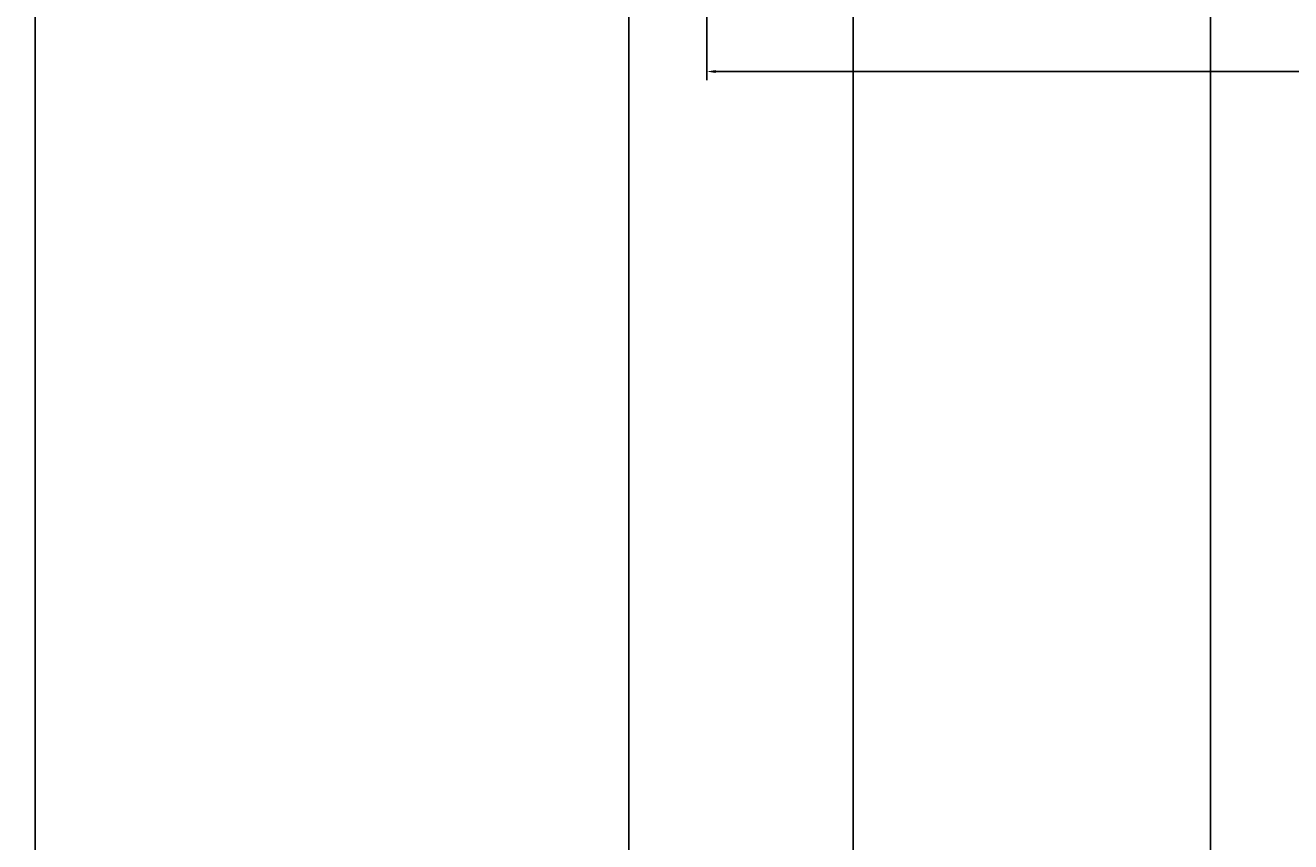
# Model space of a CAD drawing. Units: inches. Extents: x 2231 to 2461, y 2045 to 2455.
# Tile 89 of 95: x 2384 to 2410, y 2383 to 2400. Entities that reach past the tile are written whole.
import ezdxf

# ---------------------------------------------------------------- set-up
doc = ezdxf.new("R2010")
doc.units = ezdxf.units.IN
doc.layers.add('A-ANNO-DIMS', color=2, linetype='Continuous', lineweight=18)
doc.styles.get("Standard").update_dxf_attribs({"font": 'arial.ttf'})
doc.dimstyles.get("Standard").update_dxf_attribs({"dimtxt": 0.18, "dimasz": 0.18, "dimexe": 0.18, "dimexo": 0.0625, "dimgap": 0.09, "dimtad": 0, "dimtih": 1, "dimtoh": 1, "dimdec": 4, "dimzin": 0, "dimdsep": 46, "dimtxsty": 'Standard', "dimcen": 0.09, "dimadec": 0, "dimazin": 0, "dimtfac": 1, "dimtdec": 4, "dimtofl": 0, "dimtmove": 0, "dimatfit": 3, "dimfxl": 1, "dimtolj": 1, "dimtzin": 0, "dimarcsym": 0})

# ---------------------------------------------------------------- blocks, each defined once
blk = doc.blocks.new('*D21')
at = {"layer": 'A-ANNO-DIMS', "color": 0, "lineweight": -2, "transparency": 16777216}
for p, q in [((2398.404, 2404.126), (2398.404, 2399.052)), ((2431.45, 2404.126), (2431.45, 2399.052)), ((2398.584, 2399.232), (2414.46, 2399.232)), ((2431.27, 2399.232), (2415.394, 2399.232))]:
    blk.add_line(p, q, dxfattribs=at)
at = {"layer": 'A-ANNO-DIMS', "color": 0, "transparency": 16777216}
for points in [[(2398.584, 2399.262), (2398.584, 2399.202), (2398.404, 2399.232)], [(2431.27, 2399.262), (2431.27, 2399.202), (2431.45, 2399.232)]]:
    blk.add_solid(points, dxfattribs=at)
at = {"layer": 'Defpoints', "color": 0, "transparency": 16777216}
for p in [(2398.404, 2404.189), (2431.45, 2404.189), (2431.45, 2399.232)]:
    blk.add_point(p, dxfattribs=at)
at = {"layer": 'A-ANNO-DIMS', "color": 0, "transparency": 16777216, "insert": (2414.927, 2399.232), "char_height": 0.18, "attachment_point": 5}
blk.add_mtext('\\A1;WC 33', dxfattribs=at)
blk = doc.blocks.new('*D42')
at = {"layer": 'A-ANNO-DIMS', "color": 0, "lineweight": -2, "transparency": 16777216}
for p, q in [((2396.794, 2286.895), (2396.794, 2454.645)), ((2432.794, 2286.895), (2432.794, 2454.645)), ((2396.974, 2454.465), (2414.575, 2454.465)), ((2432.614, 2454.465), (2415.012, 2454.465))]:
    blk.add_line(p, q, dxfattribs=at)
at = {"layer": 'A-ANNO-DIMS', "color": 0, "transparency": 16777216}
for points in [[(2396.974, 2454.495), (2396.974, 2454.435), (2396.794, 2454.465)], [(2432.614, 2454.495), (2432.614, 2454.435), (2432.794, 2454.465)]]:
    blk.add_solid(points, dxfattribs=at)
at = {"layer": 'Defpoints', "color": 0, "transparency": 16777216}
for p in [(2432.794, 2454.465), (2396.794, 2286.833), (2432.794, 2286.833)]:
    blk.add_point(p, dxfattribs=at)
at = {"layer": 'A-ANNO-DIMS', "color": 0, "transparency": 16777216, "insert": (2414.794, 2454.465), "char_height": 0.18, "attachment_point": 5}
blk.add_mtext('\\A1;36', dxfattribs=at)
blk = doc.blocks.new('*D59')
at = {"layer": 'A-ANNO-DIMS', "color": 0, "lineweight": -2, "transparency": 16777216}
for p, q in [((2408.794, 2182.895), (2408.794, 2454.645)), ((2432.794, 2182.895), (2432.794, 2454.645)), ((2408.974, 2454.465), (2420.573, 2454.465)), ((2432.614, 2454.465), (2421.014, 2454.465))]:
    blk.add_line(p, q, dxfattribs=at)
at = {"layer": 'A-ANNO-DIMS', "color": 0, "transparency": 16777216}
for points in [[(2408.974, 2454.495), (2408.974, 2454.435), (2408.794, 2454.465)], [(2432.614, 2454.495), (2432.614, 2454.435), (2432.794, 2454.465)]]:
    blk.add_solid(points, dxfattribs=at)
at = {"layer": 'Defpoints', "color": 0, "transparency": 16777216}
for p in [(2432.794, 2454.465), (2408.794, 2182.833), (2432.794, 2182.833)]:
    blk.add_point(p, dxfattribs=at)
at = {"layer": 'A-ANNO-DIMS', "color": 0, "transparency": 16777216, "insert": (2420.794, 2454.465), "char_height": 0.18, "attachment_point": 5}
blk.add_mtext('\\A1;24', dxfattribs=at)
blk = doc.blocks.new('*D66')
at = {"layer": 'A-ANNO-DIMS', "color": 0, "lineweight": -2, "transparency": 16777216}
for p, q in [((2348.189, 2096.895), (2348.189, 2454.645)), ((2408.794, 2096.895), (2408.794, 2454.645)), ((2348.369, 2454.465), (2378.167, 2454.465)), ((2408.614, 2454.465), (2378.815, 2454.465))]:
    blk.add_line(p, q, dxfattribs=at)
at = {"layer": 'A-ANNO-DIMS', "color": 0, "transparency": 16777216}
for points in [[(2348.369, 2454.495), (2348.369, 2454.435), (2348.189, 2454.465)], [(2408.614, 2454.495), (2408.614, 2454.435), (2408.794, 2454.465)]]:
    blk.add_solid(points, dxfattribs=at)
at = {"layer": 'Defpoints', "color": 0, "transparency": 16777216}
for p in [(2408.794, 2454.465), (2348.189, 2096.833), (2408.794, 2096.833)]:
    blk.add_point(p, dxfattribs=at)
at = {"layer": 'A-ANNO-DIMS', "color": 0, "transparency": 16777216, "insert": (2378.491, 2454.465), "char_height": 0.18, "attachment_point": 5}
blk.add_mtext('\\A1;60.6', dxfattribs=at)
blk = doc.blocks.new('*D71')
at = {"layer": 'A-ANNO-DIMS', "color": 0, "lineweight": -2, "transparency": 16777216}
for p, q in [((2401.422, 2092.979), (2401.422, 2454.645)), ((2408.794, 2096.895), (2408.794, 2454.645)), ((2401.602, 2454.465), (2404.732, 2454.465)), ((2408.614, 2454.465), (2405.483, 2454.465))]:
    blk.add_line(p, q, dxfattribs=at)
at = {"layer": 'A-ANNO-DIMS', "color": 0, "transparency": 16777216}
for points in [[(2401.602, 2454.495), (2401.602, 2454.435), (2401.422, 2454.465)], [(2408.614, 2454.495), (2408.614, 2454.435), (2408.794, 2454.465)]]:
    blk.add_solid(points, dxfattribs=at)
at = {"layer": 'Defpoints', "color": 0, "transparency": 16777216}
for p in [(2408.794, 2454.465), (2408.794, 2096.833), (2401.422, 2092.917)]:
    blk.add_point(p, dxfattribs=at)
at = {"layer": 'A-ANNO-DIMS', "color": 0, "transparency": 16777216, "insert": (2405.108, 2454.465), "char_height": 0.18, "attachment_point": 5}
blk.add_mtext('\\A1;7.371', dxfattribs=at)
blk = doc.blocks.new('*D72')
at = {"layer": 'A-ANNO-DIMS', "color": 0, "lineweight": -2, "transparency": 16777216}
for p, q in [((2384.543, 2145.12), (2384.543, 2454.645)), ((2408.794, 2150.677), (2408.794, 2454.645)), ((2384.723, 2454.465), (2396.272, 2454.465)), ((2408.614, 2454.465), (2397.064, 2454.465))]:
    blk.add_line(p, q, dxfattribs=at)
at = {"layer": 'A-ANNO-DIMS', "color": 0, "transparency": 16777216}
for points in [[(2384.723, 2454.495), (2384.723, 2454.435), (2384.543, 2454.465)], [(2408.614, 2454.495), (2408.614, 2454.435), (2408.794, 2454.465)]]:
    blk.add_solid(points, dxfattribs=at)
at = {"layer": 'Defpoints', "color": 0, "transparency": 16777216}
for p in [(2408.794, 2454.465), (2408.794, 2150.615), (2384.543, 2145.058)]:
    blk.add_point(p, dxfattribs=at)
at = {"layer": 'A-ANNO-DIMS', "color": 0, "transparency": 16777216, "insert": (2396.668, 2454.465), "char_height": 0.18, "attachment_point": 5}
blk.add_mtext('\\A1;24.25', dxfattribs=at)

msp = doc.modelspace()

# ---------------------------------------------------------------- dimensions: what is measured, and where the dimension line sits
at = {"layer": 'A-ANNO-DIMS'}
for base, p1, p2, override, picture, middle in [((2408.7935, 2454.4653), (2348.1888, 2096.8328), (2408.7935, 2096.8328), {"dimdec": 1, "dimlfac": 1, "dimrnd": 0, "dimzin": 0, "dimdsep": 46, "dimlunit": 2}, '*D66', (2378.4912, 2454.4653)), ((2408.7935, 2454.4653), (2384.5428, 2145.0576), (2408.7935, 2150.6145), {"dimdec": 2, "dimlfac": 1, "dimrnd": 0, "dimzin": 0, "dimdsep": 46, "dimlunit": 2}, '*D72', (2396.6682, 2454.4653)), ((2432.7935, 2454.4653), (2396.7935, 2286.8328), (2432.7935, 2286.8328), {"dimdec": 0, "dimlfac": 1, "dimrnd": 0, "dimzin": 0, "dimdsep": 46, "dimlunit": 2}, '*D42', (2414.7935, 2454.4653)), ((2408.7935, 2454.4653), (2401.4221, 2092.9167), (2408.7935, 2096.8328), {"dimdec": 3, "dimlfac": 1, "dimrnd": 0, "dimzin": 0, "dimdsep": 46, "dimlunit": 2}, '*D71', (2405.1078, 2454.4653)), ((2432.7935, 2454.4653), (2408.7935, 2182.8328), (2432.7935, 2182.8328), {"dimdec": 0, "dimlfac": 1, "dimrnd": 0, "dimzin": 0, "dimdsep": 46, "dimlunit": 2}, '*D59', (2420.7935, 2454.4653))]:
    dim = msp.add_linear_dim(base=base, p1=p1, p2=p2, dimstyle='Standard', override=override, dxfattribs=at)
    dim.commit()
    dim.dimension.update_dxf_attribs({"geometry": picture, "text_midpoint": middle})
dim = msp.add_linear_dim(base=(2431.4505, 2399.2319), p1=(2398.4042, 2404.1888), p2=(2431.4505, 2404.1888), text='WC <>', dimstyle='Standard', override={"dimdec": 0, "dimlfac": 1, "dimrnd": 0, "dimzin": 0, "dimdsep": 46, "dimlunit": 2}, dxfattribs=at)
dim.commit()
dim.dimension.update_dxf_attribs({"geometry": '*D21', "text_midpoint": (2414.9274, 2399.2319)})

doc.saveas('drawing.dxf')
